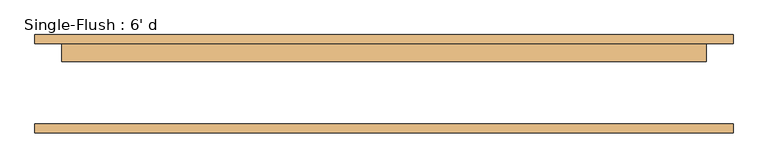
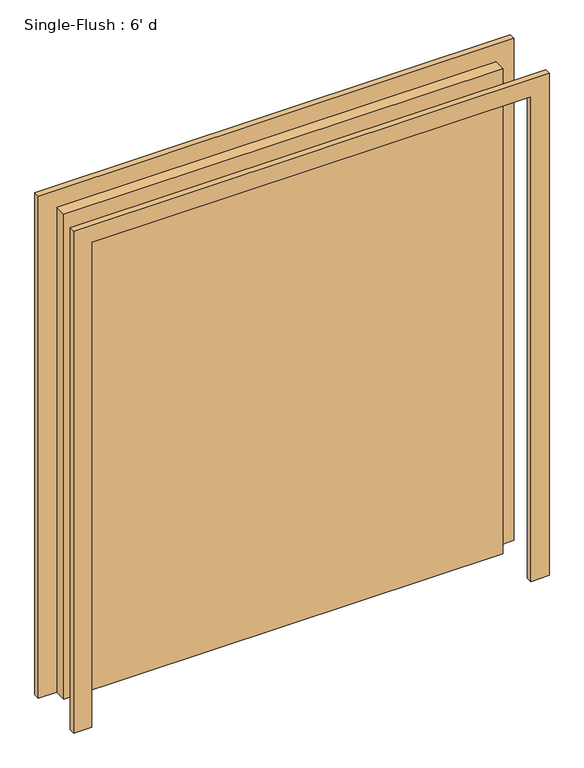
"""IFC4 building model written with IfcOpenShell, lengths in millimetres: door geometry, Single-Flush : 6' d."""

from ifc_helpers import new_model, si_unit, frame, origin, origin_with_axes, place, context, project, spatial, polyline, outline, extrude, source, transform, mapped, element, save


def single_flush_6_d_bd5e0b13(model_context):
    return source(origin(), model_context, "Body", "SweptSolid", [
        extrude(outline(polyline([(2209.8, -990.6), (0.0, -990.6), (0.0, -914.4), (2133.6, -914.4), (2133.6, 914.4), (0.0, 914.4), (0.0, 990.6), (2209.8, 990.6), (2209.8, -990.6)])), frame((0.0, 114.3, 0.0), z_axis=(0.0, 1.0, 0.0), x_axis=(0.0, 0.0, 1.0)), (0.0, 0.0, 1.0), 25.4),
        extrude(outline(polyline([(2209.8, 990.6), (2209.8, -990.6), (0.0, -990.6), (0.0, -914.4), (2133.6, -914.4), (2133.6, 914.4), (0.0, 914.4), (0.0, 990.6), (2209.8, 990.6)])), frame((0.0, -139.7, 0.0), z_axis=(0.0, 1.0, 0.0), x_axis=(0.0, 0.0, 1.0)), (0.0, 0.0, 1.0), 25.4),
        extrude(outline(polyline([(914.4, 63.5), (-914.4, 63.5), (-914.4, 114.3), (914.4, 114.3), (914.4, 63.5)])), origin_with_axes(), (0.0, 0.0, 1.0), 2133.6),
    ])


if __name__ == "__main__":
    model = new_model("IFC4")
    model_context = context("Model", 3, world=origin())
    ifc_project = project(units=[si_unit("LENGTHUNIT", "METRE", prefix="MILLI")], contexts=[model_context])
    site = spatial("IfcSite", under=ifc_project)
    building = spatial("IfcBuilding", under=site)
    placement = place(None, origin())
    single_flush_6_d_shape = single_flush_6_d_bd5e0b13(model_context)
    element("IfcDoor", 1, ObjectType="Single-Flush : 6' d", at=placement, inside=building, context=model_context, shape_type="MappedRepresentation", body=[
        mapped(single_flush_6_d_shape, transform((0.0, 0.0, 0.0), x_axis=(1.0, 0.0, 0.0), y_axis=(0.0, 1.0, 0.0), z_axis=(0.0, 0.0, 1.0))),
    ])
    save(model, "model.ifc")

# Revit data of these elements
# Type "Single-Flush : 6' d"
#   Type Mark = "12"
#   Construction Type Id = "MDOOR"
#   Assembly Code = "C1020"
#   Analytic Construction = "Metal"
#   Thickness = 0' - 2"
#   Heat Transfer Coefficient (U) = 0.651978 BTU/(h·ft²·°F)
#   Height = 7' - 0"
#   Trim Projection Ext = 0' - 1"
#   Trim Projection Int = 0' - 1"
#   Trim Width = 0' - 3"
#   Width = 6' - 0"
#   Define Thermal Properties by = 1
#   Door Material = Door - Panel
#   Frame Material = Door - Frame
#   Visual Light Transmittance = 0
#   Solar Heat Gain Coefficient = 0
#   Function = (empty or 0)
#   Wall Closure = (empty or 0)
# Element 1 (IfcDoor, "Single-Flush : 6' d")
#   Materials on its faces: "Door - Frame", "Door - Panel"
# Materials
#   "Door - Panel": class "Wood", colour RGB 210 159 95, transparency 0, Cost = 0
#   "Door - Frame": colour RGB 118 70 51, transparency 0, Cost = 0
